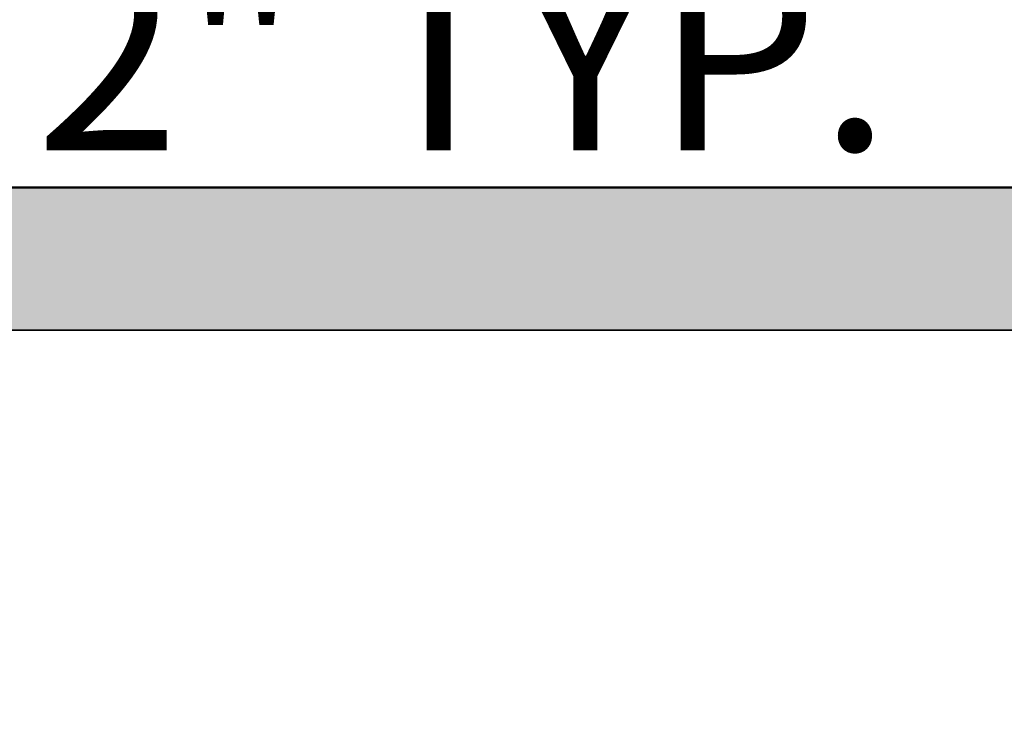
# Model space of a CAD drawing. Units: inches. Extents: x 2083 to 3317, y 1141 to 2115.
# Tile 119 of 256: x 3006 to 3068, y 1238 to 1283. Entities that reach past the tile are written whole.
import ezdxf

# ---------------------------------------------------------------- set-up
doc = ezdxf.new("R2010")
doc.units = ezdxf.units.IN
doc.layers.add('A-ANNO-DIMS', color=2, linetype='Continuous', lineweight=18)
doc.layers.add('A-WALL', color=7, linetype='Continuous', lineweight=35)
doc.layers.add('A-WALL-PATT', color=251, linetype='Continuous', lineweight=13, true_color=0x636466)
doc.styles.get("Standard").update_dxf_attribs({"font": 'arial.ttf'})
doc.dimstyles.new('ISO-25', dxfattribs={"dimtxt": 12, "dimasz": 12, "dimexe": 1.25, "dimexo": 0.625, "dimtad": 1, "dimlunit": 3, "dimtxsty": 'Standard', "dimcen": 2.5, "dimadec": 0, "dimazin": 0, "dimtfac": 1, "dimtmove": 0, "dimatfit": 3, "dimfxl": 1, "dimarcsym": 0})

# ---------------------------------------------------------------- blocks, each defined once
blk = doc.blocks.new('*D10')
at = {"layer": 'A-ANNO-DIMS', "color": 0, "lineweight": -2, "transparency": 16777216}
for p, q in [((2862.96, 1262.636), (2862.96, 1201.384)), ((3126.96, 1262.636), (3126.96, 1201.384)), ((2874.96, 1202.634), (3114.96, 1202.634))]:
    blk.add_line(p, q, dxfattribs=at)
at = {"layer": 'A-ANNO-DIMS', "color": 0, "transparency": 16777216}
for points in [[(2874.96, 1204.634), (2874.96, 1200.634), (2862.96, 1202.634)], [(3114.96, 1204.634), (3114.96, 1200.634), (3126.96, 1202.634)]]:
    blk.add_solid(points, dxfattribs=at)
at = {"layer": 'Defpoints', "color": 0, "transparency": 16777216}
for p in [(2862.96, 1263.261), (3126.96, 1263.261), (3126.96, 1202.634)]:
    blk.add_point(p, dxfattribs=at)
at = {"layer": 'A-ANNO-DIMS', "color": 0, "transparency": 16777216, "insert": (2994.96, 1209.284), "char_height": 12, "attachment_point": 5}
blk.add_mtext("22'", dxfattribs=at)
blk = doc.blocks.new('*D26')
at = {"layer": 'A-ANNO-DIMS', "color": 0, "lineweight": -2, "transparency": 16777216}
for p, q in [((3088.986, 1274.915), (3088.986, 1270.952)), ((3111.24, 1274.915), (3111.24, 1270.952)), ((3076.986, 1272.202), (2840.262, 1272.202)), ((3111.24, 1272.202), (3088.986, 1272.202)), ((3123.24, 1272.202), (3135.24, 1272.202))]:
    blk.add_line(p, q, dxfattribs=at)
at = {"layer": 'A-ANNO-DIMS', "color": 0, "transparency": 16777216}
for points in [[(3076.986, 1274.202), (3076.986, 1270.202), (3088.986, 1272.202)], [(3123.24, 1274.202), (3123.24, 1270.202), (3111.24, 1272.202)]]:
    blk.add_solid(points, dxfattribs=at)
at = {"layer": 'Defpoints', "color": 0, "transparency": 16777216}
for p in [(3088.986, 1275.54), (3111.24, 1275.54), (3088.986, 1272.202)]:
    blk.add_point(p, dxfattribs=at)
at = {"layer": 'A-ANNO-DIMS', "color": 0, "transparency": 16777216, "insert": (2952.624, 1279.032), "char_height": 12, "attachment_point": 5}
blk.add_mtext('NIGHTSTAND 1\'-10 1/2" TYP.', dxfattribs=at)
blk = doc.blocks.new('*D34')
at = {"layer": 'A-ANNO-DIMS', "color": 0, "lineweight": -2, "transparency": 16777216}
for p, q in [((2226.96, 1262.636), (2226.96, 1209.661)), ((3126.96, 1262.636), (3126.96, 1209.661)), ((2238.96, 1210.911), (3114.96, 1210.911))]:
    blk.add_line(p, q, dxfattribs=at)
at = {"layer": 'A-ANNO-DIMS', "color": 0, "transparency": 16777216}
for points in [[(2238.96, 1212.911), (2238.96, 1208.911), (2226.96, 1210.911)], [(3114.96, 1212.911), (3114.96, 1208.911), (3126.96, 1210.911)]]:
    blk.add_solid(points, dxfattribs=at)
at = {"layer": 'Defpoints', "color": 0, "transparency": 16777216}
for p in [(2226.96, 1263.261), (3126.96, 1263.261), (3126.96, 1210.911)]:
    blk.add_point(p, dxfattribs=at)
at = {"layer": 'A-ANNO-DIMS', "color": 0, "transparency": 16777216, "insert": (2676.96, 1217.663), "char_height": 12, "attachment_point": 5}
blk.add_mtext('75\'-0"', dxfattribs=at)

msp = doc.modelspace()

# ---------------------------------------------------------------- hatches: boundary and pattern name
at = {"layer": 'A-WALL-PATT'}
h = msp.add_hatch(color=256, dxfattribs=at)
h.dxf.hatch_style = 1
h.paths.add_polyline_path([(3126.96, 2020.761), (2748.96, 2020.761), (2604.96, 2020.761), (2226.96, 2020.761), (2226.96, 1702.761), (2466.96, 1702.761), (2466.96, 1582.761), (2418.96, 1582.761), (2418.96, 1477.761), (2226.96, 1477.761), (2226.96, 1263.261), (2544.96, 1263.261), (2544.96, 1411.761), (2604.96, 1411.761), (2685.96, 1411.761), (2685.96, 1420.761), (2604.96, 1420.761), (2604.96, 1573.761), (2604.96, 1702.761), (2604.96, 2011.761), (2748.96, 2011.761), (2748.96, 1702.761), (2862.96, 1702.761), (2862.96, 1621.761), (2871.96, 1621.761), (2871.96, 1702.761), (2883.96, 1702.761), (2883.96, 1706.939, -0.026459), (2883.96, 1711.761), (2757.96, 1711.761), (2757.96, 1807.761), (2787.96, 1807.761), (2787.96, 1812.261), (2757.96, 1812.261), (2757.96, 2011.761), (2877.96, 2011.761), (2877.96, 1812.261), (2847.96, 1812.261), (2847.96, 1807.761), (2889.836, 1807.761), (2889.836, 1812.261), (2882.46, 1812.261), (2882.46, 2011.761), (3117.96, 2011.761), (3117.96, 1812.261), (2937.836, 1812.261), (2937.836, 1807.761), (2995.71, 1807.761), (2995.71, 1796.118), (3000.21, 1796.118), (3000.21, 1807.761), (3117.96, 1807.761), (3117.96, 1711.761), (3000.21, 1711.761), (3000.21, 1760.118), (2998.573, 1760.118, -0.020711), (2995.71, 1760.118), (2995.71, 1711.761), (2931.96, 1711.761), (2931.96, 1702.761), (3126.96, 1702.761)])
h.paths.add_polyline_path([(2471.46, 2011.761), (2471.46, 1810.011), (2462.717, 1810.011), (2462.717, 1805.511), (2505.96, 1805.511), (2505.96, 1810.011), (2475.96, 1810.011), (2475.96, 2011.761), (2595.96, 2011.761), (2595.96, 1810.011), (2565.96, 1810.011), (2565.96, 1805.511), (2595.96, 1805.511), (2595.96, 1711.761), (2235.96, 1711.761), (2235.96, 1805.511), (2353.71, 1805.511), (2353.71, 1796.054), (2358.21, 1796.054), (2358.21, 1805.511), (2414.717, 1805.511), (2414.717, 1810.011), (2235.96, 1810.011), (2235.96, 2011.761)], flags=16)
h.paths.add_polyline_path([(2270.205, 1994.61), (2270.205, 1970.61), (2246.205, 1970.61), (2246.205, 1994.61)], flags=0)
edge = h.paths.add_edge_path(flags=0)
edge.add_ellipse((2332.027, 1899.798), major_axis=(-3.043, 3.043), ratio=0.168252, start_angle=-161.33217, end_angle=-156.30711, ccw=False)
edge.add_ellipse((2333.082, 1898.744), major_axis=(-1.055, 1.055), ratio=0.453532, start_angle=-123.37102, end_angle=-94.15911)
edge = h.paths.add_edge_path(flags=0)
edge.add_ellipse((2332.027, 1968.876), major_axis=(3.043, 3.043), ratio=0.168252, start_angle=18.66783, end_angle=23.69289)
edge.add_spline(control_points=[(2332.926, 1970.691), (2332.227, 1970.336), (2330.894, 1969.659), (2328.413, 1970.932), (2327.204, 1967.749), (2324.71, 1969.956), (2322.533, 1967.012), (2320.013, 1971.296), (2317.68, 1968.158), (2316.041, 1967.102), (2315.427, 1966.81)], knot_values=[0, 0, 0, 0, 2.267059, 4.324559, 6.685584, 8.878641, 11.121502, 14.300359, 17.755284, 19.732645, 19.732645, 19.732645, 19.732645], degree=3, periodic=0)
edge.add_ellipse((2332.027, 1968.876), major_axis=(3.043, 3.043), ratio=0.168252, start_angle=18.66783, end_angle=23.69289, ccw=False)
edge.add_ellipse((2333.082, 1969.931), major_axis=(1.055, 1.055), ratio=0.453532, start_angle=56.62898, end_angle=85.84089, ccw=False)
edge = h.paths.add_edge_path(flags=0)
edge.add_spline(control_points=[(2296.428, 1967.988), (2293.628, 1965.336), (2287.704, 1959.727), (2299.744, 1949.996), (2294.533, 1935.669), (2290.573, 1920.604), (2293.394, 1909.974), (2296.185, 1904.967)], knot_values=[0.099185, 0.099185, 0.099185, 0.099185, 0.345301, 0.619822, 0.982653, 1.386093, 1.810555, 1.810555, 1.810555, 1.810555], degree=3, periodic=0)
edge.add_spline(control_points=[(2296.185, 1904.967), (2297.384, 1902.619), (2298.001, 1901.949), (2298.553, 1901.468)], knot_values=[0.006246, 0.006246, 0.006246, 0.006246, 0.055476, 0.055476, 0.055476, 0.055476], degree=3, periodic=0)
edge.add_spline(control_points=[(2298.553, 1901.468), (2297.259, 1900.923), (2295.225, 1900.232), (2293.06, 1900.614), (2292.101, 1900.788), (2292.09, 1900.791)], knot_values=[0.312835, 0.312835, 0.312835, 0.312835, 0.40178, 0.474987, 0.475903, 0.475903, 0.475903, 0.475903], degree=3, periodic=0)
edge.add_arc((2292.794, 1904.664), 3.937, 215.4209, 259.69818, ccw=False)
edge.add_spline(control_points=[(2289.585, 1902.382), (2289.477, 1902.535), (2289.368, 1902.688), (2289.261, 1902.841)], knot_values=[0.102872, 0.102872, 0.102872, 0.102872, 0.116896, 0.116896, 0.116896, 0.116896], degree=3, periodic=0)
edge.add_spline(control_points=[(2289.261, 1902.841), (2288.687, 1902.55), (2287.64, 1902.02), (2285.881, 1901.874), (2283.853, 1901.504), (2281.72, 1899.711), (2278.467, 1899.493), (2276.157, 1901.883), (2272.259, 1899.804), (2267.778, 1901.843), (2262.244, 1900.184), (2257.415, 1901.782), (2254.318, 1900.726), (2253.178, 1900.337)], knot_values=[0, 0, 0, 0, 1.907977, 3.477176, 5.261074, 7.972851, 11.680248, 13.717921, 16.939592, 22.789562, 27.502503, 33.595215, 37.145618, 37.145618, 37.145618, 37.145618], degree=3, periodic=0)
edge.add_line((2253.178, 1900.337), (2250.244, 1902.841))
edge.add_line((2250.244, 1902.841), (2250.244, 1965.833))
edge.add_line((2250.244, 1965.833), (2253.178, 1968.337))
edge.add_spline(control_points=[(2253.178, 1968.337), (2254.318, 1967.948), (2257.415, 1966.892), (2262.244, 1968.49), (2267.778, 1966.831), (2271.527, 1968.537), (2273.876, 1967.828), (2274.207, 1967.728)], knot_values=[0, 0, 0, 0, 0.09018, 0.244935, 0.364644, 0.513233, 0.537855, 0.537855, 0.537855, 0.537855], degree=3, periodic=0)
edge.add_arc((2274.353, 1963.793), 3.937, 72.05113, 92.12795, ccw=False)
edge.add_arc((2281.297, 1985.23), 18.596, 252.05113, 288.56572)
edge.add_arc((2292.317, 1956.029), 12.646, 71.02679, 113.77822, ccw=False)
edge = h.paths.add_edge_path(flags=0)
edge.add_spline(control_points=[(2274.899, 1951.856), (2275.066, 1951.617), (2275.233, 1951.377), (2275.398, 1951.136)], knot_values=[1.409916, 1.409916, 1.409916, 1.409916, 1.43159, 1.43159, 1.43159, 1.43159], degree=3, periodic=0)
edge.add_spline(control_points=[(2275.398, 1951.136), (2275.792, 1950.562), (2276.179, 1949.984), (2276.546, 1949.397)], knot_values=[1.358238, 1.358238, 1.358238, 1.358238, 1.409916, 1.409916, 1.409916, 1.409916], degree=3, periodic=0)
edge.add_line((2276.546, 1949.397), (2277.437, 1947.862))
edge.add_spline(control_points=[(2277.437, 1947.862), (2276.304, 1945.673), (2274.64, 1942.427), (2274.632, 1938.094), (2272.799, 1930.852), (2274.356, 1943.897), (2275.948, 1947.923), (2276.546, 1949.397)], knot_values=[0.005632, 0.005632, 0.005632, 0.005632, 0.186014, 0.266002, 0.357087, 0.59639, 0.739732, 0.739732, 0.739732, 0.739732], degree=3, periodic=0)
edge.add_spline(control_points=[(2276.546, 1949.397), (2276.179, 1949.984), (2275.792, 1950.562), (2275.398, 1951.136)], knot_values=[1.358238, 1.358238, 1.358238, 1.358238, 1.409916, 1.409916, 1.409916, 1.409916], degree=3, periodic=0)
edge.add_spline(control_points=[(2275.398, 1951.136), (2274.943, 1950.08), (2274.208, 1948.025), (2273.935, 1944.851), (2272.469, 1937.627), (2273.466, 1945.696), (2274.701, 1951.059), (2274.899, 1951.856)], knot_values=[0.104364, 0.104364, 0.104364, 0.104364, 0.189636, 0.269624, 0.36071, 0.600013, 0.644622, 0.644622, 0.644622, 0.644622], degree=3, periodic=0)
h.paths.add_polyline_path([(2269.168, 1963.128, -0.357527), (2268.171, 1960.976, -0.092561), (2268.171, 1939.436, -0.357527), (2269.168, 1937.285, -0.357527), (2267.016, 1938.282, -0.164785), (2254.686, 1938.282, -0.357527), (2252.534, 1937.285, -0.357527), (2253.531, 1939.436, -0.092561), (2253.531, 1960.976, -0.357527), (2252.534, 1963.128, -0.357527), (2254.686, 1962.131, -0.164785), (2267.016, 1962.131, -0.357527)], flags=0)
h.paths.add_polyline_path([(2248.874, 1967.802), (2248.874, 1957.028), (2249.458, 1957.028), (2249.458, 1911.647), (2248.874, 1911.647), (2248.874, 1900.873), (2246.512, 1900.873, 0.197327), (2244.15, 1902.457), (2244.15, 1966.218, 0.197327), (2246.512, 1967.802)], flags=0)
h.paths.add_polyline_path([(2269.168, 1931.389, -0.357527), (2268.171, 1929.238, -0.092561), (2268.171, 1907.698, -0.357527), (2269.168, 1905.547, -0.357527), (2267.016, 1906.544, -0.164785), (2254.686, 1906.544, -0.357527), (2252.534, 1905.547, -0.357527), (2253.531, 1907.698, -0.092561), (2253.531, 1929.238, -0.357527), (2252.534, 1931.389, -0.357527), (2254.686, 1930.392, -0.164785), (2267.016, 1930.392, -0.357527)], flags=0)
edge = h.paths.add_edge_path(flags=0)
edge.add_spline(control_points=[(2276.197, 1906.724), (2276.168, 1909.029), (2276.114, 1913.372), (2270.598, 1924.925), (2273.905, 1919.013), (2275.922, 1916.262), (2275.475, 1912.402), (2277.258, 1910.381), (2276.696, 1908.225), (2276.646, 1906.813), (2276.618, 1906.008)], knot_values=[0, 0, 0, 0, 8.61026, 16.221274, 18.843057, 23.804898, 27.440828, 29.356102, 31.203478, 33.650687, 33.650687, 33.650687, 33.650687], degree=3, periodic=0)
edge.add_spline(control_points=[(2276.618, 1906.008), (2276.623, 1905.624), (2276.498, 1904.629), (2275.442, 1903.855), (2274.937, 1903.08), (2274.859, 1902.841)], knot_values=[0.156488, 0.156488, 0.156488, 0.156488, 0.184398, 0.231376, 0.250598, 0.250598, 0.250598, 0.250598], degree=3, periodic=0)
edge.add_line((2274.859, 1902.841), (2276.506, 1902.841))
edge.add_spline(control_points=[(2276.506, 1902.841), (2276.788, 1903.085), (2277.665, 1904.125), (2278.25, 1904.341), (2277.654, 1908.527), (2278.156, 1906.228), (2278.1, 1905.286), (2278.847, 1904.069), (2277.857, 1903.415), (2277.874, 1902.991), (2277.904, 1902.841)], knot_values=[0.059574, 0.059574, 0.059574, 0.059574, 0.080753, 0.103741, 0.16972, 0.176036, 0.207137, 0.240474, 0.262341, 0.27366, 0.27366, 0.27366, 0.27366], degree=3, periodic=0)
edge.add_line((2277.904, 1902.841), (2280.03, 1902.841))
edge.add_spline(control_points=[(2280.03, 1902.841), (2279.888, 1903.088), (2279.499, 1903.982), (2280.152, 1905.939), (2278.104, 1909.658), (2279.762, 1907.185), (2280.328, 1904.875), (2280.485, 1903.49), (2281.463, 1903.249), (2281.758, 1902.936), (2281.834, 1902.841)], knot_values=[0.013856, 0.013856, 0.013856, 0.013856, 0.034874, 0.088867, 0.107879, 0.126738, 0.158714, 0.193757, 0.217487, 0.226722, 0.226722, 0.226722, 0.226722], degree=3, periodic=0)
edge.add_spline(control_points=[(2281.834, 1902.841), (2281.788, 1902.827), (2281.647, 1902.783), (2281.396, 1902.859), (2281.088, 1902.985), (2280.721, 1903.061), (2280.333, 1903.026), (2280.125, 1902.899), (2280.03, 1902.841)], knot_values=[0, 0, 0, 0, 0.14413, 0.435517, 0.749276, 1.153046, 1.548371, 1.878348, 1.878348, 1.878348, 1.878348], degree=3, periodic=0)
edge.add_line((2280.03, 1902.841), (2277.904, 1902.841))
edge.add_spline(control_points=[(2277.904, 1902.841), (2277.893, 1902.796), (2277.865, 1902.68), (2277.607, 1902.687), (2277.274, 1902.801), (2276.838, 1902.62), (2276.584, 1902.789), (2276.506, 1902.841)], knot_values=[0, 0, 0, 0, 0.127189, 0.326199, 0.628009, 1.24357, 1.515331, 1.515331, 1.515331, 1.515331], degree=3, periodic=0)
edge.add_line((2276.506, 1902.841), (2274.859, 1902.841))
edge.add_spline(control_points=[(2274.859, 1902.841), (2274.814, 1902.899), (2274.725, 1903.013), (2274.493, 1903.119), (2274.244, 1902.961), (2273.937, 1903.185), (2273.614, 1902.983), (2273.408, 1902.883), (2273.322, 1902.841)], knot_values=[0, 0, 0, 0, 0.21843, 0.436957, 0.687977, 0.990379, 1.398396, 1.69185, 1.69185, 1.69185, 1.69185], degree=3, periodic=0)
edge.add_spline(control_points=[(2273.322, 1902.841), (2273.617, 1903.446), (2274.274, 1904.538), (2276.027, 1904.574), (2276.207, 1906.584), (2276.197, 1906.724)], knot_values=[0.012227, 0.012227, 0.012227, 0.012227, 0.059472, 0.106218, 0.134458, 0.134458, 0.134458, 0.134458], degree=3, periodic=0)
h.paths.add_polyline_path([(2270.776, 1897.79), (2270.776, 1873.79), (2246.776, 1873.79), (2246.776, 1897.79)], flags=0)
h.paths.add_polyline_path([(2353.71, 1760.005), (2353.71, 1760.054), (2358.21, 1760.054, -0.033729)], flags=0)
h.paths.add_polyline_path([(2321.819, 1737.529), (2341.995, 1737.529, -0.414214), (2343.203, 1736.321), (2343.203, 1721.021, -0.414214), (2341.995, 1719.813), (2321.819, 1719.813, -0.414214), (2320.611, 1721.021), (2320.611, 1736.321, -0.414214)], flags=0)
h.paths.add_polyline_path([(2324.235, 1736.321), (2339.579, 1736.321, -0.414214), (2341.995, 1733.905), (2341.995, 1725.45, -0.414214), (2339.579, 1723.034), (2333.681, 1723.034), (2333.845, 1722.045, -0.870646), (2335.425, 1721.826, -0.767327), (2333.923, 1721.423), (2331.291, 1721.423, -0.767327), (2329.788, 1721.826, -0.870646), (2331.368, 1722.045), (2331.533, 1723.034), (2324.235, 1723.034, -0.414214), (2321.819, 1725.45), (2321.819, 1733.905, -0.414214)], flags=0)
h.paths.add_polyline_path([(2570.484, 1928.615), (2589.684, 1928.615), (2590.169, 1928.615), (2590.169, 1904.993), (2570.484, 1904.993)], flags=0)
h.paths.add_polyline_path([(2574.447, 1927.264, -1), (2572.829, 1927.264, -1)], flags=0)
h.paths.add_polyline_path([(2573.09, 1926.941), (2573.925, 1927.776), (2574.148, 1927.553), (2573.313, 1926.718)], flags=0)
h.paths.add_polyline_path([(2578.779, 1919.73, -1), (2571.592, 1919.73, -1)], flags=0)
h.paths.add_polyline_path([(2578.385, 1919.73, -1), (2571.985, 1919.73, -1)], flags=0)
h.paths.add_polyline_path([(2331.596, 1729.476, -1), (2333.618, 1729.476, -1)], flags=0)
h.paths.add_polyline_path([(2578.034, 1927.264, -1), (2576.416, 1927.264, -1)], flags=0)
h.paths.add_polyline_path([(2576.689, 1927.531), (2576.912, 1927.754), (2577.747, 1926.919), (2577.524, 1926.696)], flags=0)
h.paths.add_polyline_path([(2578.139, 1909.86, -1), (2572.232, 1909.86, -1)], flags=0)
h.paths.add_polyline_path([(2577.745, 1909.86, -1), (2572.625, 1909.86, -1)], flags=0)
h.paths.add_polyline_path([(2583.798, 1927.264, -1), (2582.179, 1927.264, -1)], flags=0)
h.paths.add_polyline_path([(2582.719, 1927.754), (2583.554, 1926.919), (2583.331, 1926.696), (2582.496, 1927.531)], flags=0)
h.paths.add_polyline_path([(2582.496, 1927.531), (2582.719, 1927.754), (2583.554, 1926.919), (2583.331, 1926.696)], flags=0)
h.paths.add_polyline_path([(2587.739, 1920.53, -1), (2581.832, 1920.53, -1)], flags=0)
h.paths.add_polyline_path([(2587.345, 1920.53, -1), (2582.225, 1920.53, -1)], flags=0)
h.paths.add_polyline_path([(2587.385, 1927.264, -1), (2585.766, 1927.264, -1)], flags=0)
h.paths.add_polyline_path([(2586.082, 1926.98), (2586.917, 1927.815), (2587.14, 1927.593), (2586.305, 1926.758)], flags=0)
h.paths.add_polyline_path([(2588.379, 1910.66, -1), (2581.192, 1910.66, -1)], flags=0)
h.paths.add_polyline_path([(2587.985, 1910.66, -1), (2581.585, 1910.66, -1)], flags=0)
h.paths.add_polyline_path([(2417.168, 1729.478), (2437.344, 1729.478, -0.414214), (2438.552, 1728.27), (2438.552, 1712.969, -0.414214), (2437.344, 1711.761), (2417.168, 1711.761, -0.414214), (2415.96, 1712.969), (2415.96, 1728.27, -0.414214)], flags=0)
h.paths.add_polyline_path([(2419.584, 1728.27), (2434.928, 1728.27, -0.414214), (2437.344, 1725.854), (2437.344, 1717.398, -0.414214), (2434.928, 1714.983), (2429.029, 1714.983), (2429.194, 1713.994, -0.870646), (2430.774, 1713.775, -0.767327), (2429.271, 1713.372), (2426.64, 1713.372, -0.767327), (2425.137, 1713.775, -0.870646), (2426.717, 1713.994), (2426.882, 1714.983), (2419.584, 1714.983, -0.414214), (2417.168, 1717.398), (2417.168, 1725.854, -0.414214)], flags=0)
h.paths.add_polyline_path([(2419.584, 1728.27), (2434.928, 1728.27, -0.414214), (2437.344, 1725.854), (2437.344, 1717.398, -0.414214), (2434.928, 1714.983), (2429.029, 1714.983), (2428.358, 1719.009), (2427.553, 1719.009), (2426.882, 1714.983), (2419.584, 1714.983, -0.414214), (2417.168, 1717.398), (2417.168, 1725.854, -0.414214)], flags=0)
h.paths.add_polyline_path([(2426.944, 1721.425, -1), (2428.967, 1721.425, -1)], flags=0)
h.paths.add_polyline_path([(2475.96, 1702.761), (2595.96, 1702.761), (2595.96, 1582.761), (2475.96, 1582.761)], flags=16)
h.paths.add_polyline_path([(2427.96, 1573.761), (2595.96, 1573.761), (2595.96, 1468.761), (2595.96, 1420.761), (2384.46, 1420.761), (2384.46, 1468.761), (2427.96, 1468.761)], flags=16)
h.paths.add_polyline_path([(2379.96, 1468.761), (2379.96, 1420.761), (2235.96, 1420.761), (2235.96, 1468.761)], flags=16)
h.paths.add_polyline_path([(2317.816, 1466.696), (2337.992, 1466.696, -0.414214), (2339.2, 1465.488), (2339.2, 1450.187, -0.414214), (2337.992, 1448.979), (2317.816, 1448.979, -0.414214), (2316.608, 1450.187), (2316.608, 1465.488, -0.414214)], flags=0)
h.paths.add_polyline_path([(2320.232, 1465.488), (2335.576, 1465.488, -0.414214), (2337.992, 1463.072), (2337.992, 1454.616, -0.414214), (2335.576, 1452.2), (2329.677, 1452.2), (2329.842, 1451.212, -0.870646), (2331.422, 1450.992, -0.767327), (2329.92, 1450.59), (2327.288, 1450.59, -0.767327), (2325.785, 1450.992, -0.870646), (2327.365, 1451.212), (2327.53, 1452.2), (2320.232, 1452.2, -0.414214), (2317.816, 1454.616), (2317.816, 1463.072, -0.414214)], flags=0)
h.paths.add_polyline_path([(2320.232, 1465.488), (2335.576, 1465.488, -0.414214), (2337.992, 1463.072), (2337.992, 1454.616, -0.414214), (2335.576, 1452.2), (2329.677, 1452.2), (2329.006, 1456.227), (2328.201, 1456.227), (2327.53, 1452.2), (2320.232, 1452.2, -0.414214), (2317.816, 1454.616), (2317.816, 1463.072, -0.414214)], flags=0)
h.paths.add_polyline_path([(2327.593, 1458.643, -1), (2329.615, 1458.643, -1)], flags=0)
h.paths.add_polyline_path([(2244.412, 1433.34), (2241.921, 1433.34, -0.414214), (2240.018, 1435.244), (2240.018, 1440.953, -0.414211), (2241.921, 1442.856), (2244.412, 1442.856, -1.976472)], flags=0)
h.paths.add_polyline_path([(2245.357, 1434.398, -0.414214), (2245.357, 1441.799, -2.144098)], flags=0)
h.paths.add_polyline_path([(2535.96, 1416.261), (2535.96, 1272.261), (2235.96, 1272.261), (2235.96, 1416.261)], flags=16)
h.paths.add_polyline_path([(2260.12, 1384.293), (2260.12, 1362.039), (2237.865, 1362.039), (2237.865, 1384.293)], flags=0)
edge = h.paths.add_edge_path(flags=0)
edge.add_line((2318.252, 1362.093), (2318.146, 1362.001))
edge.add_ellipse((2317.445, 1360.431), major_axis=(2.822, 2.822), ratio=0.168252, start_angle=18.66783, end_angle=20.94813, ccw=False)
edge.add_ellipse((2318.423, 1361.409), major_axis=(0.978, 0.978), ratio=0.453532, start_angle=56.62898, end_angle=70.2262, ccw=False)
edge = h.paths.add_edge_path(flags=0)
edge.add_line((2319.107, 1295.571), (2319.015, 1295.677))
edge.add_ellipse((2317.445, 1296.378), major_axis=(-2.822, 2.822), ratio=0.168252, start_angle=-161.33217, end_angle=-159.05187, ccw=False)
edge.add_ellipse((2318.423, 1295.4), major_axis=(-0.978, 0.978), ratio=0.453532, start_angle=-123.37102, end_angle=-109.7738)
edge = h.paths.add_edge_path(flags=0)
edge.add_spline(control_points=[(2284.21, 1301.17), (2284.581, 1300.445), (2284.891, 1299.892), (2285.16, 1299.461)], knot_values=[0.039066, 0.039066, 0.039066, 0.039066, 0.055476, 0.055476, 0.055476, 0.055476], degree=3, periodic=0)
edge.add_line((2285.16, 1299.461), (2284.21, 1301.17))
edge = h.paths.add_edge_path(flags=0)
edge.add_line((2280.412, 1297.298), (2283.37, 1297.036))
edge.add_line((2283.37, 1297.036), (2286.406, 1297.926))
edge.add_spline(control_points=[(2286.406, 1297.926), (2285.305, 1297.463), (2284.345, 1297.129), (2283.37, 1297.036)], knot_values=[0.394369, 0.394369, 0.394369, 0.394369, 0.475903, 0.475903, 0.475903, 0.475903], degree=3, periodic=0)
edge.add_spline(control_points=[(2283.37, 1297.036), (2283.281, 1297.028), (2282.316, 1296.957), (2281.313, 1297.134), (2280.423, 1297.296), (2280.412, 1297.298)], knot_values=[0.312835, 0.312835, 0.312835, 0.312835, 0.320246, 0.393453, 0.394369, 0.394369, 0.394369, 0.394369], degree=3, periodic=0)
edge = h.paths.add_edge_path(flags=0)
edge.add_line((2284.436, 1359.607), (2280.446, 1355.328))
edge.add_line((2280.446, 1355.328), (2279.58, 1351.018))
edge.add_line((2279.58, 1351.018), (2282.413, 1346.58))
edge.add_spline(control_points=[(2282.413, 1346.58), (2283.153, 1345.589), (2284.253, 1344.029), (2284.801, 1342.387), (2284.935, 1341.806)], knot_values=[1.240098, 1.240098, 1.240098, 1.240098, 1.332892, 1.382712, 1.382712, 1.382712, 1.382712], degree=3, periodic=0)
edge.add_spline(control_points=[(2284.935, 1341.806), (2285.319, 1340.141), (2285.233, 1338.409), (2284.91, 1336.654)], knot_values=[1.097484, 1.097484, 1.097484, 1.097484, 1.240098, 1.240098, 1.240098, 1.240098], degree=3, periodic=0)
edge.add_spline(control_points=[(2284.91, 1336.654), (2284.587, 1334.899), (2284.027, 1333.12), (2283.463, 1331.361)], knot_values=[0.95487, 0.95487, 0.95487, 0.95487, 1.097484, 1.097484, 1.097484, 1.097484], degree=3, periodic=0)
edge.add_line((2283.463, 1331.361), (2281.89, 1326.153))
edge.add_line((2281.89, 1326.153), (2280.756, 1321.056))
edge.add_line((2280.756, 1321.056), (2280.299, 1316.002))
edge.add_line((2280.299, 1316.002), (2280.716, 1310.95))
edge.add_line((2280.716, 1310.95), (2282.028, 1305.972))
edge.add_line((2282.028, 1305.972), (2284.21, 1301.17))
edge.add_spline(control_points=[(2284.21, 1301.17), (2283.341, 1302.73), (2282.612, 1304.336), (2282.028, 1305.972)], knot_values=[0.099185, 0.099185, 0.099185, 0.099185, 0.241799, 0.241799, 0.241799, 0.241799], degree=3, periodic=0)
edge.add_spline(control_points=[(2282.028, 1305.972), (2281.444, 1307.608), (2281.005, 1309.273), (2280.716, 1310.95)], knot_values=[0.241799, 0.241799, 0.241799, 0.241799, 0.384413, 0.384413, 0.384413, 0.384413], degree=3, periodic=0)
edge.add_spline(control_points=[(2280.716, 1310.95), (2280.433, 1312.588), (2280.289, 1314.277), (2280.299, 1315.962), (2280.299, 1316.002)], knot_values=[0.384413, 0.384413, 0.384413, 0.384413, 0.523647, 0.527028, 0.527028, 0.527028, 0.527028], degree=3, periodic=0)
edge.add_spline(control_points=[(2280.299, 1316.002), (2280.312, 1317.687), (2280.478, 1319.368), (2280.756, 1321.056)], knot_values=[0.527028, 0.527028, 0.527028, 0.527028, 0.669642, 0.669642, 0.669642, 0.669642], degree=3, periodic=0)
edge.add_spline(control_points=[(2280.756, 1321.056), (2281.035, 1322.744), (2281.426, 1324.44), (2281.89, 1326.153)], knot_values=[0.669642, 0.669642, 0.669642, 0.669642, 0.812256, 0.812256, 0.812256, 0.812256], degree=3, periodic=0)
edge.add_spline(control_points=[(2281.89, 1326.153), (2282.264, 1327.533), (2282.788, 1329.262), (2283.353, 1331.018), (2283.463, 1331.361)], knot_values=[0.812256, 0.812256, 0.812256, 0.812256, 0.927087, 0.95487, 0.95487, 0.95487, 0.95487], degree=3, periodic=0)
edge.add_line((2283.463, 1331.361), (2284.91, 1336.654))
edge.add_line((2284.91, 1336.654), (2284.935, 1341.806))
edge.add_line((2284.935, 1341.806), (2282.413, 1346.58))
edge.add_spline(control_points=[(2282.413, 1346.58), (2281.275, 1348.104), (2280.078, 1349.57), (2279.58, 1351.018)], knot_values=[1.382712, 1.382712, 1.382712, 1.382712, 1.525326, 1.525326, 1.525326, 1.525326], degree=3, periodic=0)
edge.add_spline(control_points=[(2279.58, 1351.018), (2279.443, 1351.415), (2279.136, 1352.857), (2279.735, 1354.29), (2280.446, 1355.328)], knot_values=[1.525326, 1.525326, 1.525326, 1.525326, 1.564439, 1.667941, 1.667941, 1.667941, 1.667941], degree=3, periodic=0)
edge.add_spline(control_points=[(2280.446, 1355.328), (2281.426, 1356.758), (2282.931, 1358.183), (2284.436, 1359.607)], knot_values=[1.667941, 1.667941, 1.667941, 1.667941, 1.810555, 1.810555, 1.810555, 1.810555], degree=3, periodic=0)
edge.add_arc((2280.623, 1348.518), 11.726, 71.02679, 113.77822)
edge.add_arc((2270.405, 1375.595), 17.244, 252.05113, 288.56572, ccw=False)
edge.add_arc((2263.966, 1355.718), 3.651, 72.05113, 92.12795)
edge.add_arc((2263.966, 1355.718), 3.651, 92.12795, 177.98513)
edge.add_spline(control_points=[(2260.318, 1355.846), (2260.26, 1354.221), (2260.551, 1350.187), (2262.999, 1346.766), (2264.473, 1344.649)], knot_values=[1.43159, 1.43159, 1.43159, 1.43159, 1.564144, 1.770695, 1.770695, 1.770695, 1.770695], degree=3, periodic=0)
edge.add_line((2264.473, 1344.649), (2264.936, 1343.983))
edge.add_spline(control_points=[(2263.801, 1340.248), (2263.843, 1340.514), (2264.067, 1341.756), (2264.513, 1343.002), (2264.935, 1343.981)], knot_values=[0.53657, 0.53657, 0.53657, 0.53657, 0.559349, 0.644622, 0.644622, 0.644622, 0.644622], degree=3, periodic=0)
edge.add_spline(control_points=[(2264.935, 1343.981), (2265.118, 1343.715), (2265.299, 1343.448), (2265.477, 1343.179)], knot_values=[1.384077, 1.384077, 1.384077, 1.384077, 1.409916, 1.409916, 1.409916, 1.409916], degree=3, periodic=0)
edge.add_spline(control_points=[(2265.477, 1343.179), (2265.655, 1342.911), (2265.829, 1342.641), (2265.999, 1342.369)], knot_values=[1.358238, 1.358238, 1.358238, 1.358238, 1.384077, 1.384077, 1.384077, 1.384077], degree=3, periodic=0)
edge.add_line((2265.999, 1342.369), (2266.826, 1340.946))
edge.add_spline(control_points=[(2266.826, 1340.946), (2268.894, 1337.09), (2271.398, 1325.843), (2270.516, 1310.569), (2275.919, 1301.861), (2277.79, 1299.199)], knot_values=[0.116896, 0.116896, 0.116896, 0.116896, 0.472987, 1.050969, 1.313793, 1.313793, 1.313793, 1.313793], degree=3, periodic=0)
edge.add_spline(control_points=[(2277.79, 1299.199), (2277.839, 1299.128), (2277.889, 1299.057), (2277.94, 1298.987)], knot_values=[0.109884, 0.109884, 0.109884, 0.109884, 0.116896, 0.116896, 0.116896, 0.116896], degree=3, periodic=0)
edge.add_line((2277.94, 1298.987), (2277.789, 1299.199))
edge.add_spline(control_points=[(2277.789, 1299.199), (2277.257, 1298.929), (2276.286, 1298.438), (2275.039, 1298.334), (2274.383, 1298.239), (2274.215, 1298.209)], knot_values=[33.12187, 33.12187, 33.12187, 33.12187, 35.029056, 36.598255, 37.144827, 37.144827, 37.144827, 37.144827], degree=3, periodic=0)
edge.add_line((2274.215, 1298.209), (2273.073, 1297.893))
edge.add_spline(control_points=[(2273.073, 1297.893), (2272.323, 1297.58), (2271.039, 1296.511), (2269.248, 1296.226), (2268.423, 1296.375)], knot_values=[26.532584, 26.532584, 26.532584, 26.532584, 29.198919, 31.839101, 31.839101, 31.839101, 31.839101], degree=3, periodic=0)
edge.add_line((2268.423, 1296.375), (2263.879, 1297.458))
edge.add_spline(control_points=[(2263.879, 1297.458), (2263.556, 1297.359), (2261.86, 1296.839), (2260.239, 1297.282), (2258.933, 1297.516)], knot_values=[15.919551, 15.919551, 15.919551, 15.919551, 16.939592, 21.226067, 21.226067, 21.226067, 21.226067], degree=3, periodic=0)
edge.add_line((2258.933, 1297.516), (2254.055, 1297.329))
edge.add_spline(control_points=[(2254.055, 1297.329), (2253.756, 1297.296), (2252.114, 1297.165), (2250.462, 1297.544), (2249.13, 1297.668)], knot_values=[5.306517, 5.306517, 5.306517, 5.306517, 6.276435, 10.613034, 10.613034, 10.613034, 10.613034], degree=3, periodic=0)
edge.add_line((2249.13, 1297.668), (2244.332, 1296.878))
edge.add_line((2244.332, 1296.878), (2241.611, 1299.199))
edge.add_line((2241.611, 1299.199), (2241.611, 1357.609))
edge.add_line((2241.611, 1357.609), (2244.332, 1359.931))
edge.add_line((2244.332, 1359.931), (2252.729, 1359.543))
edge.add_spline(control_points=[(2252.729, 1359.543), (2252.871, 1359.546), (2253.306, 1359.548), (2253.74, 1359.514), (2254.032, 1359.482)], knot_values=[0.233291, 0.233291, 0.233291, 0.233291, 0.244935, 0.268927, 0.268927, 0.268927, 0.268927], degree=3, periodic=0)
edge.add_line((2254.032, 1359.482), (2259.587, 1359.416))
edge.add_spline(control_points=[(2259.587, 1359.416), (2260.677, 1359.629), (2262.073, 1359.897), (2263.524, 1359.459), (2263.83, 1359.366)], knot_values=[0.422516, 0.422516, 0.422516, 0.422516, 0.513233, 0.537855, 0.537855, 0.537855, 0.537855], degree=3, periodic=0)
edge.add_arc((2263.966, 1355.718), 3.651, 72.05113, 92.12795, ccw=False)
edge.add_arc((2270.405, 1375.595), 17.244, 252.05113, 288.56572)
edge.add_arc((2280.623, 1348.518), 11.726, 71.02679, 113.77822, ccw=False)
h.paths.add_polyline_path([(2240.341, 1359.435), (2240.341, 1349.444), (2240.882, 1349.444), (2240.882, 1307.365), (2240.341, 1307.365), (2240.341, 1297.374), (2238.15, 1297.374, 0.197327), (2235.96, 1298.843), (2235.96, 1357.966, 0.197327), (2238.15, 1359.435)], flags=0)
h.paths.add_polyline_path([(2259.158, 1355.101, -0.357527), (2258.233, 1353.106, -0.092561), (2258.233, 1333.133, -0.357527), (2259.158, 1331.138, -0.357527), (2257.163, 1332.062, -0.164785), (2245.729, 1332.062, -0.357527), (2243.735, 1331.138, -0.357527), (2244.659, 1333.133, -0.092561), (2244.659, 1353.106, -0.357527), (2243.735, 1355.101, -0.357527), (2245.729, 1354.176, -0.164785), (2257.163, 1354.176, -0.357527)], flags=0)
edge = h.paths.add_edge_path(flags=0)
edge.add_line((2265.999, 1342.369), (2266.826, 1340.946))
edge.add_line((2266.826, 1340.946), (2265.308, 1337.814))
edge.add_line((2265.308, 1337.814), (2264.358, 1334.653))
edge.add_line((2264.358, 1334.653), (2264.262, 1333.8))
edge.add_spline(control_points=[(2264.262, 1333.8), (2264.208, 1333.187), (2264.162, 1332.366), (2264.007, 1331.414), (2263.969, 1331.202)], knot_values=[0.464444, 0.464444, 0.464444, 0.464444, 0.516691, 0.531608, 0.531608, 0.531608, 0.531608], degree=3, periodic=0)
edge.add_spline(control_points=[(2263.969, 1331.202), (2263.775, 1330.119), (2263.424, 1328.791), (2263.257, 1328.531), (2263.234, 1328.515)], knot_values=[0.372682, 0.372682, 0.372682, 0.372682, 0.44885, 0.464444, 0.464444, 0.464444, 0.464444], degree=3, periodic=0)
edge.add_spline(control_points=[(2263.234, 1328.515), (2263.096, 1328.42), (2263.131, 1329.301), (2263.275, 1330.616)], knot_values=[0.280919, 0.280919, 0.280919, 0.280919, 0.372682, 0.372682, 0.372682, 0.372682], degree=3, periodic=0)
edge.add_spline(control_points=[(2263.275, 1330.616), (2263.419, 1331.93), (2263.672, 1333.677), (2263.97, 1335.315)], knot_values=[0.189157, 0.189157, 0.189157, 0.189157, 0.280919, 0.280919, 0.280919, 0.280919], degree=3, periodic=0)
edge.add_spline(control_points=[(2263.97, 1335.315), (2264.1, 1336.032), (2264.419, 1337.622), (2264.755, 1338.864), (2264.947, 1339.491)], knot_values=[0.097394, 0.097394, 0.097394, 0.097394, 0.137578, 0.189157, 0.189157, 0.189157, 0.189157], degree=3, periodic=0)
edge.add_spline(control_points=[(2264.947, 1339.491), (2265.29, 1340.606), (2265.644, 1341.494), (2265.999, 1342.369)], knot_values=[0.005632, 0.005632, 0.005632, 0.005632, 0.097394, 0.097394, 0.097394, 0.097394], degree=3, periodic=0)
h.paths.add_polyline_path([(2259.158, 1325.671, -0.357527), (2258.233, 1323.676, -0.092561), (2258.233, 1303.703, -0.357527), (2259.158, 1301.708, -0.357527), (2257.163, 1302.633, -0.164785), (2245.729, 1302.633, -0.357527), (2243.735, 1301.708, -0.357527), (2244.659, 1303.703, -0.092561), (2244.659, 1323.676, -0.357527), (2243.735, 1325.671, -0.357527), (2245.729, 1324.747, -0.164785), (2257.163, 1324.747, -0.357527)], flags=0)
edge = h.paths.add_edge_path(flags=0)
edge.add_spline(control_points=[(2261.709, 1317.311), (2261.679, 1317.418), (2261.762, 1317.389), (2262.491, 1316.09), (2262.962, 1315.301)], knot_values=[14.955861, 14.955861, 14.955861, 14.955861, 16.221274, 18.694826, 18.694826, 18.694826, 18.694826], degree=3, periodic=0)
edge.add_spline(control_points=[(2262.962, 1315.301), (2262.99, 1315.254), (2263.702, 1314.067), (2264.349, 1313.127), (2264.73, 1312.164)], knot_values=[18.694826, 18.694826, 18.694826, 18.694826, 18.843057, 22.433791, 22.433791, 22.433791, 22.433791], degree=3, periodic=0)
edge.add_spline(control_points=[(2264.73, 1312.164), (2264.876, 1311.796), (2265.177, 1310.77), (2265.143, 1309.559), (2265.248, 1308.824)], knot_values=[22.433791, 22.433791, 22.433791, 22.433791, 23.804898, 26.172756, 26.172756, 26.172756, 26.172756], degree=3, periodic=0)
edge.add_line((2265.248, 1308.824), (2265.851, 1307.172))
edge.add_spline(control_points=[(2265.851, 1307.172), (2266.065, 1306.822), (2266.384, 1306.332), (2266.424, 1305.781), (2266.42, 1305.611)], knot_values=[28.062562, 28.062562, 28.062562, 28.062562, 29.356102, 29.911721, 29.911721, 29.911721, 29.911721], degree=3, periodic=0)
edge.add_spline(control_points=[(2266.42, 1305.611), (2266.416, 1305.433), (2266.394, 1305.25), (2266.365, 1305.066)], knot_values=[29.911721, 29.911721, 29.911721, 29.911721, 30.497837, 30.497837, 30.497837, 30.497837], degree=3, periodic=0)
edge.add_line((2266.365, 1305.066), (2266.066, 1302.136))
edge.add_spline(control_points=[(2266.066, 1302.136), (2266.071, 1301.78), (2265.998, 1301.2), (2265.663, 1300.759), (2265.509, 1300.586)], knot_values=[0.156488, 0.156488, 0.156488, 0.156488, 0.184398, 0.203543, 0.203543, 0.203543, 0.203543], degree=3, periodic=0)
edge.add_line((2265.509, 1300.586), (2264.435, 1299.199))
edge.add_line((2264.435, 1299.199), (2265.962, 1299.199))
edge.add_line((2265.962, 1299.199), (2267.336, 1301.175))
edge.add_line((2267.336, 1301.175), (2267.312, 1301.986))
edge.add_spline(control_points=[(2267.312, 1301.986), (2267.261, 1302.862), (2267.16, 1303.737), (2267.271, 1303.326)], knot_values=[0.126229, 0.126229, 0.126229, 0.126229, 0.166617, 0.166617, 0.166617, 0.166617], degree=3, periodic=0)
edge.add_spline(control_points=[(2267.271, 1303.326), (2267.28, 1303.294), (2267.31, 1303.175), (2267.373, 1302.884), (2267.406, 1302.683), (2267.418, 1302.601)], knot_values=[0.166617, 0.166617, 0.166617, 0.166617, 0.16972, 0.176036, 0.180765, 0.180765, 0.180765, 0.180765], degree=3, periodic=0)
edge.add_spline(control_points=[(2267.744, 1300.988), (2267.688, 1301.151), (2267.481, 1301.657), (2267.484, 1302.145), (2267.418, 1302.601)], knot_values=[0.180765, 0.180765, 0.180765, 0.180765, 0.193767, 0.220139, 0.220139, 0.220139, 0.220139], degree=3, periodic=0)
edge.add_line((2267.418, 1302.601), (2267.744, 1300.988))
edge.add_spline(control_points=[(2267.744, 1300.988), (2267.832, 1300.732), (2267.932, 1300.31), (2267.555, 1299.975), (2267.429, 1299.829)], knot_values=[0.220139, 0.220139, 0.220139, 0.220139, 0.240474, 0.25489, 0.25489, 0.25489, 0.25489], degree=3, periodic=0)
edge.add_line((2267.429, 1299.829), (2267.258, 1299.199))
edge.add_line((2267.258, 1299.199), (2269.23, 1299.199))
edge.add_spline(control_points=[(2269.23, 1299.199), (2269.099, 1299.429), (2268.843, 1300.016), (2269.012, 1300.916), (2268.947, 1301.661)], knot_values=[0.013856, 0.013856, 0.013856, 0.013856, 0.034874, 0.067073, 0.067073, 0.067073, 0.067073], degree=3, periodic=0)
edge.add_line((2268.947, 1301.661), (2268.432, 1303.603))
edge.add_spline(control_points=[(2268.432, 1303.603), (2268.176, 1304.192), (2267.596, 1305.251), (2268.041, 1304.623), (2268.251, 1304.282)], knot_values=[0.090155, 0.090155, 0.090155, 0.090155, 0.107879, 0.120289, 0.120289, 0.120289, 0.120289], degree=3, periodic=0)
edge.add_spline(control_points=[(2268.251, 1304.282), (2268.361, 1304.105), (2269.058, 1302.918), (2269.383, 1301.59), (2269.521, 1300.776), (2269.575, 1300.556)], knot_values=[0.120289, 0.120289, 0.120289, 0.120289, 0.126738, 0.158714, 0.173506, 0.173506, 0.173506, 0.173506], degree=3, periodic=0)
edge.add_line((2269.575, 1300.556), (2270.686, 1299.421))
edge.add_spline(control_points=[(2270.686, 1299.421), (2270.767, 1299.357), (2270.838, 1299.281), (2270.903, 1299.199)], knot_values=[0.21816, 0.21816, 0.21816, 0.21816, 0.226722, 0.226722, 0.226722, 0.226722], degree=3, periodic=0)
edge.add_line((2270.937, 1299.193), (2270.903, 1299.199))
edge.add_spline(control_points=[(2270.903, 1299.199), (2270.86, 1299.186), (2270.73, 1299.146), (2270.496, 1299.216), (2270.272, 1299.308), (2270.121, 1299.348), (2270.063, 1299.36)], knot_values=[0.939174, 0.939174, 0.939174, 0.939174, 1.083304, 1.374691, 1.68845, 1.878348, 1.878348, 1.878348, 1.878348], degree=3, periodic=0)
edge.add_line((2270.063, 1299.36), (2269.23, 1299.199))
edge.add_line((2269.23, 1299.199), (2267.258, 1299.199))
edge.add_spline(control_points=[(2267.258, 1299.199), (2267.248, 1299.157), (2267.223, 1299.05), (2266.984, 1299.057), (2266.809, 1299.116), (2266.677, 1299.109), (2266.637, 1299.105)], knot_values=[0.757665, 0.757665, 0.757665, 0.757665, 0.884854, 1.083864, 1.385675, 1.515331, 1.515331, 1.515331, 1.515331], degree=3, periodic=0)
edge.add_spline(control_points=[(2266.637, 1299.105), (2266.485, 1299.089), (2266.236, 1299.017), (2266.035, 1299.151), (2265.962, 1299.199)], knot_values=[0, 0, 0, 0, 0.485905, 0.757665, 0.757665, 0.757665, 0.757665], degree=3, periodic=0)
edge.add_line((2265.962, 1299.199), (2264.435, 1299.199))
edge.add_line((2264.435, 1299.199), (2263.858, 1299.367))
edge.add_spline(control_points=[(2263.858, 1299.367), (2263.819, 1299.371), (2263.78, 1299.386), (2263.74, 1299.402)], knot_values=[0.845925, 0.845925, 0.845925, 0.845925, 0.978627, 0.978627, 0.978627, 0.978627], degree=3, periodic=0)
edge.add_line((2263.722, 1299.396), (2263.01, 1299.199))
edge.add_spline(control_points=[(2263.01, 1299.199), (2263.246, 1299.683), (2263.506, 1300.128), (2263.873, 1300.408)], knot_values=[0.012227, 0.012227, 0.012227, 0.012227, 0.052971, 0.052971, 0.052971, 0.052971], degree=3, periodic=0)
edge.add_spline(control_points=[(2263.873, 1300.408), (2263.932, 1300.453), (2264.084, 1300.553), (2264.255, 1300.624), (2264.36, 1300.665)], knot_values=[0.052971, 0.052971, 0.052971, 0.052971, 0.059472, 0.069086, 0.069086, 0.069086, 0.069086], degree=3, periodic=0)
edge.add_line((2264.36, 1300.665), (2265.142, 1301.078))
edge.add_line((2265.142, 1301.078), (2265.676, 1302.8))
edge.add_line((2265.676, 1302.8), (2265.541, 1305.704))
edge.add_line((2265.541, 1305.704), (2264.803, 1309.328))
edge.add_line((2264.803, 1309.328), (2263.041, 1314.092))
edge.add_spline(control_points=[(2263.041, 1314.092), (2262.384, 1315.671), (2261.796, 1316.998), (2261.709, 1317.311)], knot_values=[11.216896, 11.216896, 11.216896, 11.216896, 14.955861, 14.955861, 14.955861, 14.955861], degree=3, periodic=0)
h.paths.add_polyline_path([(2871.96, 1416.261), (2895.91, 1416.261), (2895.91, 1420.761), (2871.96, 1420.761), (2871.96, 1501.761), (2862.96, 1501.761), (2862.96, 1420.761), (2805.96, 1420.761), (2805.96, 1411.761), (2862.96, 1411.761), (2862.96, 1263.261), (3126.96, 1263.261), (3126.96, 1411.761), (3126.96, 1486.761), (2943.96, 1486.761), (2943.96, 1477.761), (2967.86, 1477.761), (2967.86, 1420.761), (2943.91, 1420.761), (2943.91, 1416.261), (3117.96, 1416.261), (3117.96, 1420.761), (2972.36, 1420.761), (2972.36, 1477.761), (3117.96, 1477.761), (3117.96, 1420.761), (3117.96, 1272.261), (2871.96, 1272.261)], flags=0)
h.paths.add_polyline_path([(2457.126, 1485.943), (2527.603, 1485.943), (2527.603, 1537.636), (2457.126, 1537.636)], flags=8)
h.paths.add_polyline_path([(2481.005, 1609.982), (2590.766, 1609.982), (2590.766, 1682.003), (2481.005, 1682.003)], flags=8)
h.paths.add_polyline_path([(2483.085, 1729.127), (2553.562, 1729.127), (2553.562, 1780.82), (2483.085, 1780.82)], flags=8)
h = msp.add_hatch(color=256, dxfattribs=at)
h.dxf.hatch_style = 1
h.paths.add_polyline_path([(3126.96, 1486.761), (2943.96, 1486.761), (2943.96, 1477.761), (2967.86, 1477.761), (2967.86, 1420.761), (2943.91, 1420.761), (2943.91, 1416.261), (3117.96, 1416.261), (3117.96, 1420.761), (2972.36, 1420.761), (2972.36, 1477.761), (3117.96, 1477.761), (3117.96, 1420.761), (3117.96, 1272.261), (2871.96, 1272.261), (2871.96, 1416.261), (2895.91, 1416.261), (2895.91, 1420.761), (2871.96, 1420.761), (2871.96, 1501.761), (2862.96, 1501.761), (2862.96, 1420.761), (2805.96, 1420.761), (2805.96, 1411.761), (2862.96, 1411.761), (2862.96, 1263.261), (3126.96, 1263.261), (3126.96, 1411.761)])

# ---------------------------------------------------------------- linework, layer by layer
at = {"layer": 'A-WALL'}
for p, q in [((2871.96, 1272.261), (3117.96, 1272.261)), ((2544.96, 1263.261), (3126.96, 1263.261))]:
    msp.add_line(p, q, dxfattribs=at)

# ---------------------------------------------------------------- dimensions: what is measured, and where the dimension line sits
at = {"layer": 'A-ANNO-DIMS'}
dim = msp.add_linear_dim(base=(3088.986, 1272.202), p1=(3111.24, 1275.54), p2=(3088.986, 1275.54), angle=180, text='NIGHTSTAND <> TYP.', dimstyle='ISO-25', override={"dimdec": 1, "dimlfac": 1, "dimrnd": 0, "dimzin": 1, "dimdsep": 46, "dimlunit": 4, "dimfrac": 2}, dxfattribs=at)
dim.commit()
dim.dimension.update_dxf_attribs({"geometry": '*D26', "text_midpoint": (2952.624, 1279.032)})
for base, p1, override, picture, middle in [((3126.96, 1210.911), (2226.96, 1263.261), {"dimdec": 1, "dimlfac": 1, "dimrnd": 0, "dimzin": 1, "dimdsep": 46, "dimlunit": 4, "dimfrac": 2}, '*D34', (2676.96, 1217.663)), ((3126.96, 1202.634), (2862.96, 1263.261), {"dimclrd": 0, "dimclre": 0, "dimclrt": 0}, '*D10', (2994.96, 1209.284))]:
    dim = msp.add_linear_dim(base=base, p1=p1, p2=(3126.96, 1263.261), dimstyle='ISO-25', override=override, dxfattribs=at)
    dim.commit()
    dim.dimension.update_dxf_attribs({"geometry": picture, "text_midpoint": middle})

doc.saveas('drawing.dxf')
